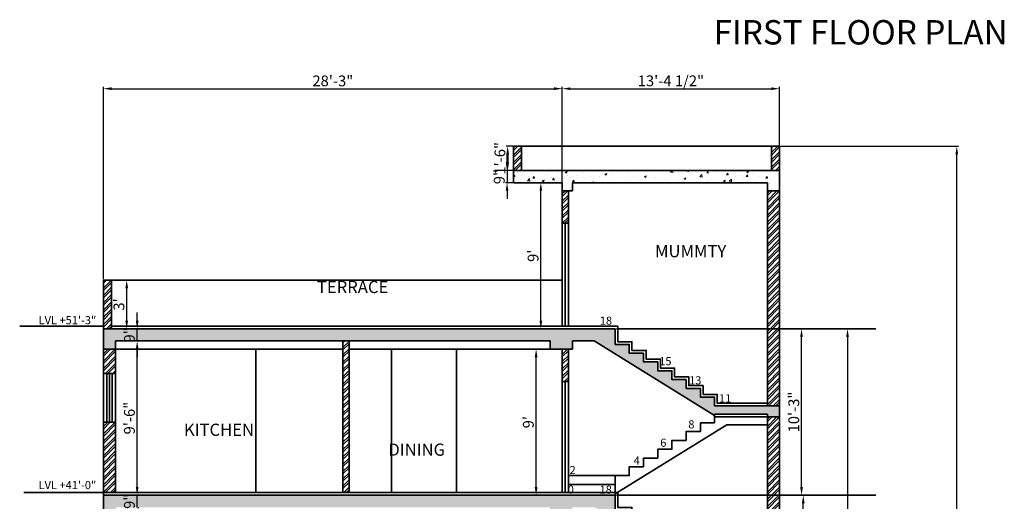
# Model space of a CAD drawing. Units: millimetres. Extents: x 1706 to 5913, y 156 to 1716.
# Tile 20 of 26: x 4414 to 5141, y 693 to 1049. Entities that reach past the tile are written whole.
import ezdxf

# ---------------------------------------------------------------- set-up
doc = ezdxf.new("R2010")
doc.units = ezdxf.units.MM
for name, color, linetype, lineweight in [('A-ANNO-DIMS', 2, 'Continuous', 18), ('A-ANNO-SYMB', 3, 'Continuous', 18), ('A-ANNO-TEXT', 7, 'Continuous', 18), ('A-AREA-IDEN', 3, 'Continuous', 18), ('A-SECT', 7, 'Continuous', 35), ('A-SECT-PATT', 8, 'Continuous', 13)]:
    doc.layers.add(name, color=color, linetype=linetype, lineweight=lineweight)
doc.styles.get("Standard").update_dxf_attribs({"font": 'arial.ttf'})
doc.dimstyles.new('ISO-25', dxfattribs={"dimtxt": 8, "dimasz": 6, "dimexe": 1.25, "dimexo": 0.625, "dimtad": 1, "dimdec": 0, "dimlunit": 3, "dimtxsty": 'Standard', "dimcen": 2.5, "dimadec": 0, "dimazin": 0, "dimtfac": 1, "dimtdec": 0, "dimtmove": 0, "dimatfit": 3, "dimfxl": 1, "dimarcsym": 0})
pattern_1 = [(45, (229.4607, 1496.8062), (-2.6940768, 2.6940768), []), (45, (231.2567, 1496.8062), (-2.6940768, 2.6940768), [])]
pattern_2 = [(50, (229.461, 1496.806), (14.574774, -1.275127), [1.524, -16.764]), (355, (229.46, 1496.806), (-2.819474, 15.284548), [1.2192, -13.411247]), (100.45144, (230.675, 1496.7), (11.7553, 14.00942), [1.2952, -14.24722]), (46.1842, (229.46, 1500.87), (21.68632, -3.363386), [2.286, -25.146]), (96.63556, (231.268, 1500.59), (18.99233, 19.79409), [1.9428, -21.37085]), (351.18415, (229.46, 1500.87), (18.99233, 19.79409), [1.8288, -20.11678]), (21, (231.493, 1499.854), (12.12915, -8.181216), [1.524, -16.764]), (326, (231.493, 1499.854), (4.94416, 14.735037), [1.2192, -13.4112]), (71.45144, (232.503, 1499.172), (17.073314, 6.55382), [1.2952, -14.247195]), (37.5, (229.4607, 1496.806), (0.247088, 6.764403), [0, -13.24864, 0, -13.6144, 0, -13.462]), (7.5, (229.461, 1496.806), (5.345573, 8.014446), [0, -7.76224, 0, -12.94384, 0, -5.1308]), (327.5, (224.9293, 1496.806), (10.8472476, -0.4582995), [0, -5.08, 0, -15.8496, 0, -21.0312]), (317.5, (222.897, 1496.806), (11.850335, 2.03412), [0, -6.604, 0, -10.52576, 0, -14.9352])]

# ---------------------------------------------------------------- blocks, each defined once
blk = doc.blocks.new('*D177')
at = {"layer": 'A-ANNO-DIMS', "color": 0, "lineweight": -2, "transparency": 16777216}
for p, q in [((4500.87, 703.75), (4500.87, 709.75)), ((4500.87, 688.75), (4500.87, 697.75)), ((4501.49, 697.75), (4502.12, 697.75)), ((4501.49, 688.75), (4502.12, 688.75)), ((4500.87, 682.75), (4500.87, 676.75))]:
    blk.add_line(p, q, dxfattribs=at)
at = {"layer": 'A-ANNO-DIMS', "color": 0, "transparency": 16777216}
for points in [[(4499.87, 703.75), (4501.87, 703.75), (4500.87, 697.75)], [(4499.87, 682.75), (4501.87, 682.75), (4500.87, 688.75)]]:
    blk.add_solid(points, dxfattribs=at)
at = {"layer": 'Defpoints', "color": 0, "transparency": 16777216}
for p in [(4500.87, 697.75), (4500.87, 697.75), (4500.87, 688.75)]:
    blk.add_point(p, dxfattribs=at)
at = {"layer": 'A-ANNO-DIMS', "color": 0, "transparency": 16777216, "insert": (4496.16, 693.25), "char_height": 8, "attachment_point": 5, "rotation": 90}
blk.add_mtext('9"', dxfattribs=at)
blk = doc.blocks.new('*D178')
at = {"layer": 'A-ANNO-DIMS', "color": 0, "lineweight": -2, "transparency": 16777216}
for p, q in [((4501.49, 811.75), (4502.12, 811.75)), ((4500.87, 703.75), (4500.87, 805.75)), ((4501.49, 697.75), (4502.12, 697.75))]:
    blk.add_line(p, q, dxfattribs=at)
at = {"layer": 'A-ANNO-DIMS', "color": 0, "transparency": 16777216}
for points in [[(4499.87, 805.75), (4501.87, 805.75), (4500.87, 811.75)], [(4499.87, 703.75), (4501.87, 703.75), (4500.87, 697.75)]]:
    blk.add_solid(points, dxfattribs=at)
at = {"layer": 'Defpoints', "color": 0, "transparency": 16777216}
for p in [(4500.87, 811.75), (4500.87, 811.75), (4500.87, 697.75)]:
    blk.add_point(p, dxfattribs=at)
at = {"layer": 'A-ANNO-DIMS', "color": 0, "transparency": 16777216, "insert": (4496.16, 754.75), "char_height": 8, "attachment_point": 5, "rotation": 90}
blk.add_mtext('9\'-6"', dxfattribs=at)
blk = doc.blocks.new('*D179')
at = {"layer": 'A-ANNO-DIMS', "color": 0, "lineweight": -2, "transparency": 16777216}
for p, q in [((4500.87, 826.75), (4500.87, 832.75)), ((4500.87, 811.75), (4500.87, 820.75)), ((4501.49, 820.75), (4502.12, 820.75)), ((4501.49, 811.75), (4502.12, 811.75)), ((4500.87, 805.75), (4500.87, 799.75))]:
    blk.add_line(p, q, dxfattribs=at)
at = {"layer": 'A-ANNO-DIMS', "color": 0, "transparency": 16777216}
for points in [[(4499.87, 826.75), (4501.87, 826.75), (4500.87, 820.75)], [(4499.87, 805.75), (4501.87, 805.75), (4500.87, 811.75)]]:
    blk.add_solid(points, dxfattribs=at)
at = {"layer": 'Defpoints', "color": 0, "transparency": 16777216}
for p in [(4500.87, 820.75), (4500.87, 820.75), (4500.87, 811.75)]:
    blk.add_point(p, dxfattribs=at)
at = {"layer": 'A-ANNO-DIMS', "color": 0, "transparency": 16777216, "insert": (4496.16, 816.25), "char_height": 8, "attachment_point": 5, "rotation": 90}
blk.add_mtext('9"', dxfattribs=at)
blk = doc.blocks.new('*D183')
at = {"layer": 'A-ANNO-DIMS', "color": 0, "lineweight": -2, "transparency": 16777216}
for p, q in [((4799.02, 805.75), (4794.34, 805.75)), ((4795.59, 703.75), (4795.59, 799.75)), ((4799.02, 697.75), (4794.34, 697.75))]:
    blk.add_line(p, q, dxfattribs=at)
at = {"layer": 'A-ANNO-DIMS', "color": 0, "transparency": 16777216}
for points in [[(4794.59, 799.75), (4796.59, 799.75), (4795.59, 805.75)], [(4794.59, 703.75), (4796.59, 703.75), (4795.59, 697.75)]]:
    blk.add_solid(points, dxfattribs=at)
at = {"layer": 'Defpoints', "color": 0, "transparency": 16777216}
for p in [(4795.59, 805.75), (4799.64, 805.75), (4799.64, 697.75)]:
    blk.add_point(p, dxfattribs=at)
at = {"layer": 'A-ANNO-DIMS', "color": 0, "transparency": 16777216, "insert": (4790.88, 751.75), "char_height": 8, "attachment_point": 5, "rotation": 90}
blk.add_mtext("9'", dxfattribs=at)
blk = doc.blocks.new('*D184')
at = {"layer": 'A-ANNO-DIMS', "color": 0, "lineweight": -2, "transparency": 16777216}
for p, q in [((4799.36, 928.75), (4800.34, 928.75)), ((4799.09, 826.75), (4799.09, 922.75)), ((4799.36, 820.75), (4800.34, 820.75))]:
    blk.add_line(p, q, dxfattribs=at)
at = {"layer": 'A-ANNO-DIMS', "color": 0, "transparency": 16777216}
for points in [[(4798.09, 922.75), (4800.09, 922.75), (4799.09, 928.75)], [(4798.09, 826.75), (4800.09, 826.75), (4799.09, 820.75)]]:
    blk.add_solid(points, dxfattribs=at)
at = {"layer": 'Defpoints', "color": 0, "transparency": 16777216}
for p in [(4798.74, 928.75), (4799.09, 928.75), (4798.74, 820.75)]:
    blk.add_point(p, dxfattribs=at)
at = {"layer": 'A-ANNO-DIMS', "color": 0, "transparency": 16777216, "insert": (4794.38, 874.75), "char_height": 8, "attachment_point": 5, "rotation": 90}
blk.add_mtext("9'", dxfattribs=at)
blk = doc.blocks.new('*D185')
at = {"layer": 'A-ANNO-DIMS', "color": 0, "lineweight": -2, "transparency": 16777216}
for p, q in [((4778.28, 955.75), (4773.35, 955.75)), ((4774.6, 949.75), (4774.6, 943.75)), ((4778.28, 937.75), (4773.35, 937.75))]:
    blk.add_line(p, q, dxfattribs=at)
at = {"layer": 'A-ANNO-DIMS', "color": 0, "transparency": 16777216}
for points in [[(4773.6, 949.75), (4775.6, 949.75), (4774.6, 955.75)], [(4773.6, 943.75), (4775.6, 943.75), (4774.6, 937.75)]]:
    blk.add_solid(points, dxfattribs=at)
at = {"layer": 'Defpoints', "color": 0, "transparency": 16777216}
for p in [(4778.91, 955.75), (4774.6, 937.75), (4778.91, 937.75)]:
    blk.add_point(p, dxfattribs=at)
at = {"layer": 'A-ANNO-DIMS', "color": 0, "transparency": 16777216, "insert": (4769.89, 946.75), "char_height": 8, "attachment_point": 5, "rotation": 90}
blk.add_mtext('1\'-6"', dxfattribs=at)
blk = doc.blocks.new('*D186')
at = {"layer": 'A-ANNO-DIMS', "color": 0, "lineweight": -2, "transparency": 16777216}
for p, q in [((4774.12, 943.75), (4774.12, 949.75)), ((4778.28, 937.75), (4772.87, 937.75)), ((4774.12, 937.75), (4774.12, 928.75)), ((4778.28, 928.75), (4772.87, 928.75)), ((4774.12, 922.75), (4774.12, 916.75))]:
    blk.add_line(p, q, dxfattribs=at)
at = {"layer": 'A-ANNO-DIMS', "color": 0, "transparency": 16777216}
for points in [[(4773.12, 943.75), (4775.12, 943.75), (4774.12, 937.75)], [(4773.12, 922.75), (4775.12, 922.75), (4774.12, 928.75)]]:
    blk.add_solid(points, dxfattribs=at)
at = {"layer": 'Defpoints', "color": 0, "transparency": 16777216}
for p in [(4778.91, 937.75), (4774.12, 928.75), (4778.91, 928.75)]:
    blk.add_point(p, dxfattribs=at)
at = {"layer": 'A-ANNO-DIMS', "color": 0, "transparency": 16777216, "insert": (4769.41, 933.25), "char_height": 8, "attachment_point": 5, "rotation": 90}
blk.add_mtext('9"', dxfattribs=at)
blk = doc.blocks.new('*D187')
at = {"layer": 'A-ANNO-DIMS', "color": 0, "lineweight": -2, "transparency": 16777216}
for p, q in [((4482.53, 856.75), (4494.39, 856.75)), ((4493.14, 826.75), (4493.14, 850.75)), ((4482.53, 820.75), (4494.39, 820.75))]:
    blk.add_line(p, q, dxfattribs=at)
at = {"layer": 'A-ANNO-DIMS', "color": 0, "transparency": 16777216}
for points in [[(4492.14, 850.75), (4494.14, 850.75), (4493.14, 856.75)], [(4492.14, 826.75), (4494.14, 826.75), (4493.14, 820.75)]]:
    blk.add_solid(points, dxfattribs=at)
at = {"layer": 'Defpoints', "color": 0, "transparency": 16777216}
for p in [(4481.91, 856.75), (4493.14, 856.75), (4481.91, 820.75)]:
    blk.add_point(p, dxfattribs=at)
at = {"layer": 'A-ANNO-DIMS', "color": 0, "transparency": 16777216, "insert": (4488.43, 838.75), "char_height": 8, "attachment_point": 5, "rotation": 90}
blk.add_mtext("3'", dxfattribs=at)
blk = doc.blocks.new('*D191')
at = {"layer": 'A-ANNO-DIMS', "color": 0, "lineweight": -2, "transparency": 16777216}
for p, q in [((4993.55, 697.75), (4991.68, 697.75)), ((4992.93, 580.75), (4992.93, 691.75)), ((4993.55, 574.75), (4991.68, 574.75))]:
    blk.add_line(p, q, dxfattribs=at)
at = {"layer": 'A-ANNO-DIMS', "color": 0, "transparency": 16777216}
for points in [[(4991.93, 691.75), (4993.93, 691.75), (4992.93, 697.75)], [(4991.93, 580.75), (4993.93, 580.75), (4992.93, 574.75)]]:
    blk.add_solid(points, dxfattribs=at)
at = {"layer": 'Defpoints', "color": 0, "transparency": 16777216}
for p in [(4992.93, 697.75), (4994.18, 697.75), (4994.18, 574.75)]:
    blk.add_point(p, dxfattribs=at)
at = {"layer": 'A-ANNO-DIMS', "color": 0, "transparency": 16777216, "insert": (4988.22, 636.25), "char_height": 8, "attachment_point": 5, "rotation": 90}
blk.add_mtext('10\'-3"', dxfattribs=at)
blk = doc.blocks.new('*D192')
at = {"layer": 'A-ANNO-DIMS', "color": 0, "lineweight": -2, "transparency": 16777216}
for p, q in [((4993.55, 820.75), (4990.43, 820.75)), ((4991.68, 703.75), (4991.68, 814.75)), ((4993.55, 697.75), (4990.43, 697.75))]:
    blk.add_line(p, q, dxfattribs=at)
at = {"layer": 'A-ANNO-DIMS', "color": 0, "transparency": 16777216}
for points in [[(4990.68, 814.75), (4992.68, 814.75), (4991.68, 820.75)], [(4990.68, 703.75), (4992.68, 703.75), (4991.68, 697.75)]]:
    blk.add_solid(points, dxfattribs=at)
at = {"layer": 'Defpoints', "color": 0, "transparency": 16777216}
for p in [(4991.68, 820.75), (4994.18, 820.75), (4994.18, 697.75)]:
    blk.add_point(p, dxfattribs=at)
at = {"layer": 'A-ANNO-DIMS', "color": 0, "transparency": 16777216, "insert": (4986.97, 759.25), "char_height": 8, "attachment_point": 5, "rotation": 90}
blk.add_mtext('10\'-3"', dxfattribs=at)
blk = doc.blocks.new('*D193')
at = {"layer": 'A-ANNO-DIMS', "color": 0, "lineweight": -2, "transparency": 16777216}
for p, q in [((5021.56, 820.75), (5026.89, 820.75)), ((5025.64, 814.75), (5025.64, 211.75)), ((5021.56, 205.75), (5026.89, 205.75))]:
    blk.add_line(p, q, dxfattribs=at)
at = {"layer": 'A-ANNO-DIMS', "color": 0, "transparency": 16777216}
for points in [[(5024.64, 814.75), (5026.64, 814.75), (5025.64, 820.75)], [(5024.64, 211.75), (5026.64, 211.75), (5025.64, 205.75)]]:
    blk.add_solid(points, dxfattribs=at)
at = {"layer": 'Defpoints', "color": 0, "transparency": 16777216}
for p in [(5020.94, 820.75), (5020.94, 205.75), (5025.64, 205.75)]:
    blk.add_point(p, dxfattribs=at)
at = {"layer": 'A-ANNO-DIMS', "color": 0, "transparency": 16777216, "insert": (5020.93, 513.25), "char_height": 8, "attachment_point": 5, "rotation": 90}
blk.add_mtext('51\'-3"', dxfattribs=at)
blk = doc.blocks.new('*D251')
at = {"layer": 'A-ANNO-DIMS', "color": 0, "lineweight": -2, "transparency": 16777216}
for p, q in [((4976.03, 955.75), (5107.63, 955.75)), ((5106.38, 211.75), (5106.38, 949.75)), ((4976.03, 205.75), (5107.63, 205.75))]:
    blk.add_line(p, q, dxfattribs=at)
at = {"layer": 'A-ANNO-DIMS', "color": 0, "transparency": 16777216}
for points in [[(5105.38, 949.75), (5107.38, 949.75), (5106.38, 955.75)], [(5105.38, 211.75), (5107.38, 211.75), (5106.38, 205.75)]]:
    blk.add_solid(points, dxfattribs=at)
at = {"layer": 'Defpoints', "color": 0, "transparency": 16777216}
for p in [(4975.41, 955.75), (5106.38, 955.75), (4975.41, 205.75)]:
    blk.add_point(p, dxfattribs=at)
at = {"layer": 'A-ANNO-DIMS', "color": 0, "transparency": 16777216, "insert": (5101.67, 580.75), "char_height": 8, "attachment_point": 5, "rotation": 90}
blk.add_mtext('62\'-6"', dxfattribs=at)
blk = doc.blocks.new('*D252')
at = {"layer": 'A-ANNO-DIMS', "color": 0, "lineweight": -2, "transparency": 16777216}
for p, q in [((4475.91, 857.37), (4475.91, 999.5)), ((4481.91, 998.25), (4808.91, 998.25)), ((4814.91, 923.37), (4814.91, 999.5))]:
    blk.add_line(p, q, dxfattribs=at)
at = {"layer": 'A-ANNO-DIMS', "color": 0, "transparency": 16777216}
for points in [[(4481.91, 999.25), (4481.91, 997.25), (4475.91, 998.25)], [(4808.91, 999.25), (4808.91, 997.25), (4814.91, 998.25)]]:
    blk.add_solid(points, dxfattribs=at)
at = {"layer": 'Defpoints', "color": 0, "transparency": 16777216}
for p in [(4814.91, 998.25), (4814.91, 922.75), (4475.91, 856.75)]:
    blk.add_point(p, dxfattribs=at)
at = {"layer": 'A-ANNO-DIMS', "color": 0, "transparency": 16777216, "insert": (4645.41, 1002.96), "char_height": 8, "attachment_point": 5}
blk.add_mtext('28\'-3"', dxfattribs=at)
blk = doc.blocks.new('*D253')
at = {"layer": 'A-ANNO-DIMS', "color": 0, "lineweight": -2, "transparency": 16777216}
for p, q in [((4814.91, 923.37), (4814.91, 999.5)), ((4820.91, 998.25), (4969.41, 998.25)), ((4975.41, 956.37), (4975.41, 999.5))]:
    blk.add_line(p, q, dxfattribs=at)
at = {"layer": 'A-ANNO-DIMS', "color": 0, "transparency": 16777216}
for points in [[(4820.91, 999.25), (4820.91, 997.25), (4814.91, 998.25)], [(4969.41, 999.25), (4969.41, 997.25), (4975.41, 998.25)]]:
    blk.add_solid(points, dxfattribs=at)
at = {"layer": 'Defpoints', "color": 0, "transparency": 16777216}
for p in [(4975.41, 998.25), (4975.41, 955.75), (4814.91, 922.75)]:
    blk.add_point(p, dxfattribs=at)
at = {"layer": 'A-ANNO-DIMS', "color": 0, "transparency": 16777216, "insert": (4895.16, 1003.01), "char_height": 8, "attachment_point": 5}
blk.add_mtext('13\'-4 1/2"', dxfattribs=at)

msp = doc.modelspace()

# ---------------------------------------------------------------- hatches: boundary and pattern name
at = {"layer": 'A-SECT-PATT'}
h = msp.add_hatch(dxfattribs=at)
h.set_pattern_fill('ANSI32', color=256, scale=0.4)
h.set_pattern_definition(pattern_1)
h.paths.add_polyline_path([(4784.91, 955.75), (4778.91, 955.75), (4778.91, 937.75), (4784.91, 937.75)])
h = msp.add_hatch(dxfattribs=at)
h.set_pattern_fill('ANSI32', color=256, scale=0.4)
h.set_pattern_definition(pattern_1)
h.paths.add_polyline_path([(4975.41, 955.75), (4969.41, 955.75), (4969.41, 937.75), (4975.41, 937.75)])
h = msp.add_hatch(dxfattribs=at)
h.set_pattern_fill('AR-CONC', color=256, scale=0.08)
h.set_pattern_definition(pattern_2)
h.paths.add_polyline_path([(4975.41, 937.75), (4778.91, 937.75), (4778.91, 928.75), (4814.91, 928.75), (4814.91, 922.75), (4822.41, 922.75), (4822.41, 928.75), (4966.41, 928.75), (4966.41, 922.75), (4975.41, 922.75)])
h = msp.add_hatch(dxfattribs=at)
h.set_pattern_fill('ANSI32', color=256, scale=0.4)
h.set_pattern_definition(pattern_1)
h.paths.add_polyline_path([(4819.41, 922.75), (4814.91, 922.75), (4814.91, 898.75), (4819.41, 898.75)])
h = msp.add_hatch(dxfattribs=at)
h.set_pattern_fill('ANSI32', color=256, scale=0.4)
h.set_pattern_definition(pattern_1)
h.paths.add_polyline_path([(4975.41, 922.75), (4966.41, 922.75), (4966.41, 763.75), (4975.41, 763.75)])
h = msp.add_hatch(dxfattribs=at)
h.set_pattern_fill('ANSI32', color=256, scale=0.4)
h.set_pattern_definition(pattern_1)
h.paths.add_polyline_path([(4481.91, 856.75), (4475.91, 856.75), (4475.91, 820.75), (4481.91, 820.75)])
h = msp.add_hatch(dxfattribs=at)
h.set_pattern_fill('AR-CONC', color=256, scale=0.08)
h.set_pattern_definition(pattern_2)
h.paths.add_polyline_path([(4853.91, 820.75), (4475.91, 820.75), (4475.91, 805.75), (4484.91, 805.75), (4484.91, 811.75), (4805.91, 811.75), (4805.91, 805.75), (4822.41, 805.75), (4822.41, 811.75), (4838.47, 811.75), (4927.41, 756.69), (4927.41, 757.75), (4966.41, 757.75), (4966.41, 755.75), (4975.41, 755.75), (4975.41, 763.75), (4927.41, 763.75), (4927.41, 770.25), (4916.91, 770.25), (4916.91, 776.75), (4906.41, 776.75), (4906.41, 783.25), (4895.91, 783.25), (4895.91, 789.75), (4885.41, 789.75), (4885.41, 796.25), (4874.91, 796.25), (4874.91, 802.75), (4864.41, 802.75), (4864.41, 809.25), (4853.91, 809.25)])
h = msp.add_hatch(dxfattribs=at)
h.set_pattern_fill('ANSI32', color=256, scale=0.4)
h.set_pattern_definition(pattern_1)
h.paths.add_polyline_path([(4657.41, 811.75), (4652.91, 811.75), (4652.91, 699.75), (4657.41, 699.75)])
h = msp.add_hatch(dxfattribs=at)
h.set_pattern_fill('ANSI32', color=256, scale=0.4)
h.set_pattern_definition(pattern_1)
h.paths.add_polyline_path([(4484.91, 805.75), (4475.91, 805.75), (4475.91, 787.75), (4484.91, 787.75)])
h = msp.add_hatch(dxfattribs=at)
h.set_pattern_fill('ANSI32', color=256, scale=0.4)
h.set_pattern_definition(pattern_1)
h.paths.add_polyline_path([(4819.41, 805.75), (4814.91, 805.75), (4814.91, 781.75), (4819.41, 781.75)])
h = msp.add_hatch(dxfattribs=at)
h.set_pattern_fill('ANSI32', color=256, scale=0.4)
h.set_pattern_definition(pattern_1)
h.paths.add_polyline_path([(4484.91, 751.75), (4475.91, 751.75), (4475.91, 699.75), (4484.91, 699.75)])
h = msp.add_hatch(dxfattribs=at)
h.set_pattern_fill('ANSI32', color=256, scale=0.4)
h.set_pattern_definition(pattern_1)
h.paths.add_polyline_path([(4975.41, 755.75), (4966.41, 755.75), (4966.41, 641.25), (4975.41, 641.25)])
h = msp.add_hatch(dxfattribs=at)
h.set_pattern_fill('AR-CONC', color=256, scale=0.08)
h.set_pattern_definition(pattern_2)
h.paths.add_polyline_path([(4853.91, 697.75), (4475.91, 697.75), (4475.91, 682.75), (4484.91, 682.75), (4484.91, 688.75), (4805.91, 688.75), (4805.91, 682.75), (4822.41, 682.75), (4822.41, 688.75), (4839.28, 688.75), (4927.41, 634.19), (4927.41, 634.75), (4966.41, 634.75), (4966.41, 632.75), (4975.41, 632.75), (4975.41, 641.25), (4927.41, 641.25), (4927.41, 647.75), (4916.91, 647.75), (4916.91, 654.25), (4906.41, 654.25), (4906.41, 660.75), (4895.91, 660.75), (4895.91, 667.25), (4885.41, 667.25), (4885.41, 673.75), (4874.91, 673.75), (4874.91, 680.25), (4864.41, 680.25), (4864.41, 686.75), (4853.91, 686.75)])

# ---------------------------------------------------------------- linework, layer by layer
at = {"layer": 'A-SECT'}
for p, q in [((4778.91, 955.75), (4778.91, 928.75)), ((4778.91, 955.75), (4784.91, 955.75)), ((4784.91, 955.75), (4784.91, 937.75)), ((4784.91, 955.75), (4969.41, 955.75)), ((4969.41, 955.75), (4969.41, 937.75)), ((4969.41, 955.75), (4975.41, 955.75)), ((4975.41, 955.75), (4975.41, 205.75)), ((4778.91, 937.75), (4975.41, 937.75)), ((4778.91, 928.75), (4814.91, 928.75)), ((4814.91, 928.75), (4814.91, 822.75)), ((4822.41, 928.75), (4966.41, 928.75)), ((4822.41, 922.75), (4822.41, 928.75)), ((4966.41, 928.75), (4966.41, 763.75)), ((4814.91, 922.75), (4822.41, 922.75)), ((4819.41, 922.75), (4819.41, 822.75)), ((4966.41, 922.75), (4975.41, 922.75)), ((4814.91, 898.75), (4819.41, 898.75)), ((4817.16, 898.75), (4817.16, 822.75)), ((4475.91, 856.75), (4475.91, 205.75)), ((4475.91, 856.75), (4814.91, 856.75)), ((4481.91, 856.75), (4481.91, 820.75)), ((4475.91, 822.75), (4414.08, 822.75)), ((4475.91, 820.75), (4853.91, 820.75)), ((4854.91, 820.75), (5046.51, 820.75)), ((4484.91, 811.75), (4484.91, 699.75)), ((4484.91, 811.75), (4805.91, 811.75)), ((4652.91, 811.75), (4652.91, 699.75)), ((4657.41, 811.75), (4657.41, 699.75)), ((4805.91, 805.75), (4805.91, 811.75)), ((4822.41, 811.75), (4838.47, 811.75)), ((4822.41, 805.75), (4822.41, 811.75)), ((4927.41, 756.69), (4838.47, 811.75)), ((4475.91, 805.75), (4652.91, 805.75)), ((4588.41, 805.75), (4588.41, 699.75)), ((4657.41, 805.75), (4822.41, 805.75)), ((4688.69, 699.75), (4688.69, 805.75)), ((4736.69, 699.75), (4736.69, 805.75)), ((4814.91, 805.75), (4814.91, 699.75)), ((4819.41, 805.75), (4819.41, 699.75)), ((4475.91, 787.75), (4484.91, 787.75)), ((4478.41, 787.75), (4478.41, 751.75)), ((4480.41, 787.75), (4480.41, 751.75)), ((4482.41, 787.75), (4482.41, 751.75)), ((4814.91, 781.75), (4819.41, 781.75)), ((4817.16, 781.75), (4817.16, 699.75)), ((4927.41, 757.75), (4966.41, 757.75)), ((4927.41, 757.75), (4927.41, 751.25)), ((4966.41, 757.75), (4966.41, 641.25)), ((4475.91, 751.75), (4484.91, 751.75)), ((4936.38, 749.75), (4853.91, 698.69)), ((4927.41, 755.75), (4966.41, 755.75)), ((4936.38, 749.75), (4966.41, 749.75)), ((4966.41, 755.75), (4975.41, 755.75)), ((4853.91, 712.25), (4819.41, 712.25)), ((4853.91, 705.75), (4819.41, 705.75)), ((4853.91, 712.25), (4853.91, 697.75)), ((4475.91, 699.75), (4417.04, 699.75)), ((4475.91, 697.75), (4853.91, 697.75)), ((4854.91, 697.75), (5046.51, 697.75))]:
    msp.add_line(p, q, dxfattribs=at)
for points in [[(4966.41, 765.75), (4929.41, 765.75), (4929.41, 772.25), (4918.91, 772.25), (4918.91, 778.75), (4908.41, 778.75), (4908.41, 785.25), (4897.91, 785.25), (4897.91, 791.75), (4887.41, 791.75), (4887.41, 798.25), (4876.91, 798.25), (4876.91, 804.75), (4866.41, 804.75), (4866.41, 811.25), (4855.91, 811.25), (4855.91, 822.75), (4481.91, 822.75)], [(4975.41, 763.75), (4927.41, 763.75), (4927.41, 770.25), (4916.91, 770.25), (4916.91, 776.75), (4906.41, 776.75), (4906.41, 783.25), (4895.91, 783.25), (4895.91, 789.75), (4885.41, 789.75), (4885.41, 796.25), (4874.91, 796.25), (4874.91, 802.75), (4864.41, 802.75), (4864.41, 809.25), (4853.91, 809.25), (4853.91, 820.75)], [(4927.41, 751.25), (4916.91, 751.25), (4916.91, 744.75), (4906.41, 744.75), (4906.41, 738.25), (4895.91, 738.25), (4895.91, 731.75), (4885.41, 731.75), (4885.41, 725.25), (4874.91, 725.25), (4874.91, 718.75), (4864.41, 718.75), (4864.41, 712.25), (4853.91, 712.25)], [(4929.41, 643.25), (4929.41, 649.75), (4918.91, 649.75), (4918.91, 656.25), (4908.41, 656.25), (4908.41, 662.75), (4897.91, 662.75), (4897.91, 669.25), (4887.41, 669.25), (4887.41, 675.75), (4876.91, 675.75), (4876.91, 682.25), (4866.41, 682.25), (4866.41, 688.75), (4855.91, 688.75), (4855.91, 699.75), (4475.91, 699.75)], [(4927.41, 641.25), (4927.41, 647.75), (4916.91, 647.75), (4916.91, 654.25), (4906.41, 654.25), (4906.41, 660.75), (4895.91, 660.75), (4895.91, 667.25), (4885.41, 667.25), (4885.41, 673.75), (4874.91, 673.75), (4874.91, 680.25), (4864.41, 680.25), (4864.41, 686.75), (4853.91, 686.75), (4853.91, 697.75)]]:
    msp.add_lwpolyline(points, dxfattribs=at)
msp.add_lwpolyline([(4475.91, 787.75), (4484.91, 787.75), (4484.91, 751.75), (4475.91, 751.75)], close=True, dxfattribs=at)

# ---------------------------------------------------------------- texts
at = {"layer": 'A-ANNO-SYMB', "char_height": 6, "attachment_point": 1}
for s, insert in [('      LVL +51\'-3"', (4417.04, 830.13)), ('      LVL +41\'-0"', (4417.04, 708.27))]:
    msp.add_mtext_dynamic_manual_height_columns(s, width=67.9131, gutter_width=12.5, heights=[0], dxfattribs=dict(at, insert=insert))
at = {"layer": 'A-ANNO-TEXT', "attachment_point": 1}
for s, width, insert, char_height in [('FIRST FLOOR PLAN', 352.5721, (4926.77, 1048.93), 18), (' 18', 13.3033, (4840.78, 829.75), 6), (' 15', 13.3033, (4884.68, 799.83), 6), (' 13', 13.3033, (4906.74, 785.67), 6), (' 11', 13.3033, (4928.86, 772.39), 6), (' 8', 13.3033, (4906.15, 753.16), 6), (' 6', 13.3033, (4885.46, 739.55), 6), (' 4', 13.3033, (4865.85, 726.38), 6), (' 2', 13.3033, (4818.45, 719.37), 6), (' 0', 13.3033, (4817.15, 704.98), 6), (' 18', 13.3033, (4840.6, 704.88), 6)]:
    msp.add_mtext_dynamic_manual_height_columns(s, width=width, gutter_width=12.5, heights=[0], dxfattribs=dict(at, insert=insert, char_height=char_height))
at = {"layer": 'A-AREA-IDEN', "char_height": 9, "attachment_point": 1}
for s, insert in [('   MUMMTY', (4875.19, 882.66)), ('   TERRACE', (4625.42, 856.18)), ('     KITCHEN', (4521.66, 750.65)), ('     DINING', (4672.68, 735.95))]:
    msp.add_mtext_dynamic_manual_height_columns(s, width=67.9131, gutter_width=12.5, heights=[0], dxfattribs=dict(at, insert=insert))

# ---------------------------------------------------------------- dimensions: what is measured, and where the dimension line sits
at = {"layer": 'A-ANNO-DIMS'}
for base, p1, p2, picture, middle in [((4975.41, 998.25), (4814.91, 922.75), (4975.41, 955.75), '*D253', (4895.16, 1003.01)), ((4814.91, 998.25), (4475.91, 856.75), (4814.91, 922.75), '*D252', (4645.41, 1002.96))]:
    dim = msp.add_linear_dim(base=base, p1=p1, p2=p2, dimstyle='ISO-25', override={"dimdec": 1, "dimlfac": 1, "dimrnd": 0, "dimzin": 1, "dimdsep": 46, "dimlunit": 4, "dimfrac": 2}, dxfattribs=at)
    dim.commit()
    dim.dimension.update_dxf_attribs({"geometry": picture, "text_midpoint": middle})
for base, p1, p2, picture, middle in [((4774.6, 937.75), (4778.91, 955.75), (4778.91, 937.75), '*D185', (4774.6, 946.75)), ((4774.12, 928.75), (4778.91, 937.75), (4778.91, 928.75), '*D186', (4774.12, 933.25)), ((4500.87, 820.75), (4500.87, 811.75), (4500.87, 820.75), '*D179', (4500.87, 816.25)), ((4500.87, 697.75), (4500.87, 688.75), (4500.87, 697.75), '*D177', (4500.87, 693.25))]:
    dim = msp.add_linear_dim(base=base, p1=p1, p2=p2, angle=90, dimstyle='ISO-25', override={"dimclrd": 0, "dimclre": 0, "dimclrt": 0}, dxfattribs=at)
    dim.commit()
    dim.dimension.update_dxf_attribs({"geometry": picture, "text_midpoint": middle, "dimtype": 160})
for base, p1, p2, override, picture, middle in [((5106.38, 955.75), (4975.41, 205.75), (4975.41, 955.75), {"dimdec": 1, "dimlfac": 1, "dimrnd": 0, "dimzin": 1, "dimdsep": 46, "dimlunit": 4, "dimfrac": 2}, '*D251', (5101.67, 580.75)), ((4799.09, 928.75), (4798.74, 820.75), (4798.74, 928.75), {"dimclrd": 0, "dimclre": 0, "dimclrt": 0}, '*D184', (4794.38, 874.75)), ((4493.14, 856.75), (4481.91, 820.75), (4481.91, 856.75), {"dimclrd": 0, "dimclre": 0, "dimclrt": 0}, '*D187', (4488.43, 838.75)), ((4991.68, 820.75), (4994.18, 697.75), (4994.18, 820.75), {"dimclrd": 0, "dimclre": 0, "dimclrt": 0}, '*D192', (4986.97, 759.25)), ((5025.64, 205.75), (5020.94, 820.75), (5020.94, 205.75), {"dimclrd": 0, "dimclre": 0, "dimclrt": 0}, '*D193', (5020.93, 513.25)), ((4500.87, 811.75), (4500.87, 697.75), (4500.87, 811.75), {"dimclrd": 0, "dimclre": 0, "dimclrt": 0}, '*D178', (4496.16, 754.75)), ((4795.59, 805.75), (4799.64, 697.75), (4799.64, 805.75), {"dimclrd": 0, "dimclre": 0, "dimclrt": 0}, '*D183', (4790.88, 751.75)), ((4992.93, 697.75), (4994.18, 574.75), (4994.18, 697.75), {"dimclrd": 0, "dimclre": 0, "dimclrt": 0}, '*D191', (4988.22, 636.25))]:
    dim = msp.add_linear_dim(base=base, p1=p1, p2=p2, angle=90, dimstyle='ISO-25', override=override, dxfattribs=at)
    dim.commit()
    dim.dimension.update_dxf_attribs({"geometry": picture, "text_midpoint": middle})

doc.saveas('drawing.dxf')
